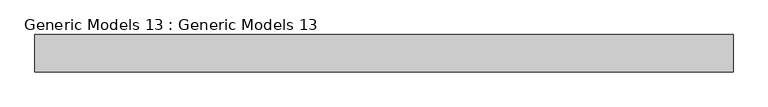
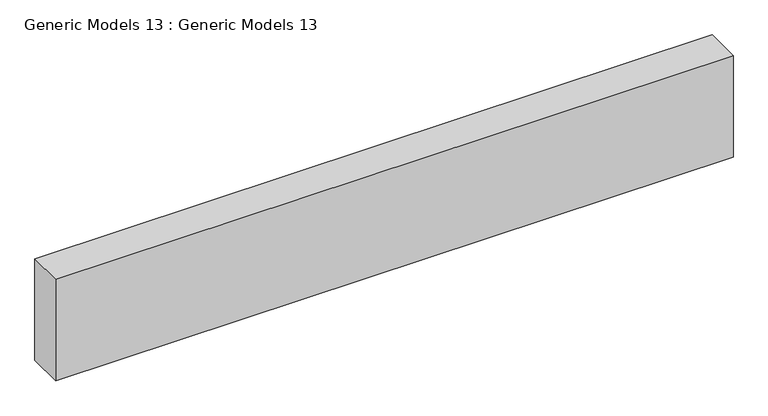
"""IFC4 building model written with IfcOpenShell, lengths in millimetres: proxy geometry, Generic Models 13 : Generic Models 13."""

from ifc_helpers import new_model, si_unit, frame, origin, place, context, project, spatial, polyline, outline, extrude, source, transform, mapped, element, save


def generic_models_13_generic_models_13_3d13953a(model_context):
    return source(origin(), model_context, "Body", "SweptSolid", [
        extrude(outline(polyline([(9958.5973594, -3927.8342514), (9958.5973594, -4842.2342514), (-7217.603092, -4842.2342514), (-7217.603092, -3927.8342514), (9958.5973594, -3927.8342514)])), frame((0.0, 0.0, 32060.000775), z_axis=(0.0, 0.0, 1.0), x_axis=(1.0, 0.0, 0.0)), (0.0, 0.0, 1.0), 2722.1399393),
    ])


if __name__ == "__main__":
    model = new_model("IFC4")
    model_context = context("Model", 3, world=origin())
    ifc_project = project(units=[si_unit("LENGTHUNIT", "METRE", prefix="MILLI")], contexts=[model_context])
    site = spatial("IfcSite", under=ifc_project)
    building = spatial("IfcBuilding", under=site)
    placement = place(None, origin())
    generic_models_13_generic_models_13_shape = generic_models_13_generic_models_13_3d13953a(model_context)
    element("IfcBuildingElementProxy", 1, Name="Generic Models 13 : Generic Models 13", ObjectType="Generic Models 13 : Generic Models 13", at=placement, inside=building, context=model_context, shape_type="MappedRepresentation", body=[
        mapped(generic_models_13_generic_models_13_shape, transform((0.0, 0.0, 0.0), x_axis=(1.0, 0.0, 0.0), y_axis=(0.0, 1.0, 0.0), z_axis=(0.0, 0.0, 1.0))),
    ])
    save(model, "model.ifc")
